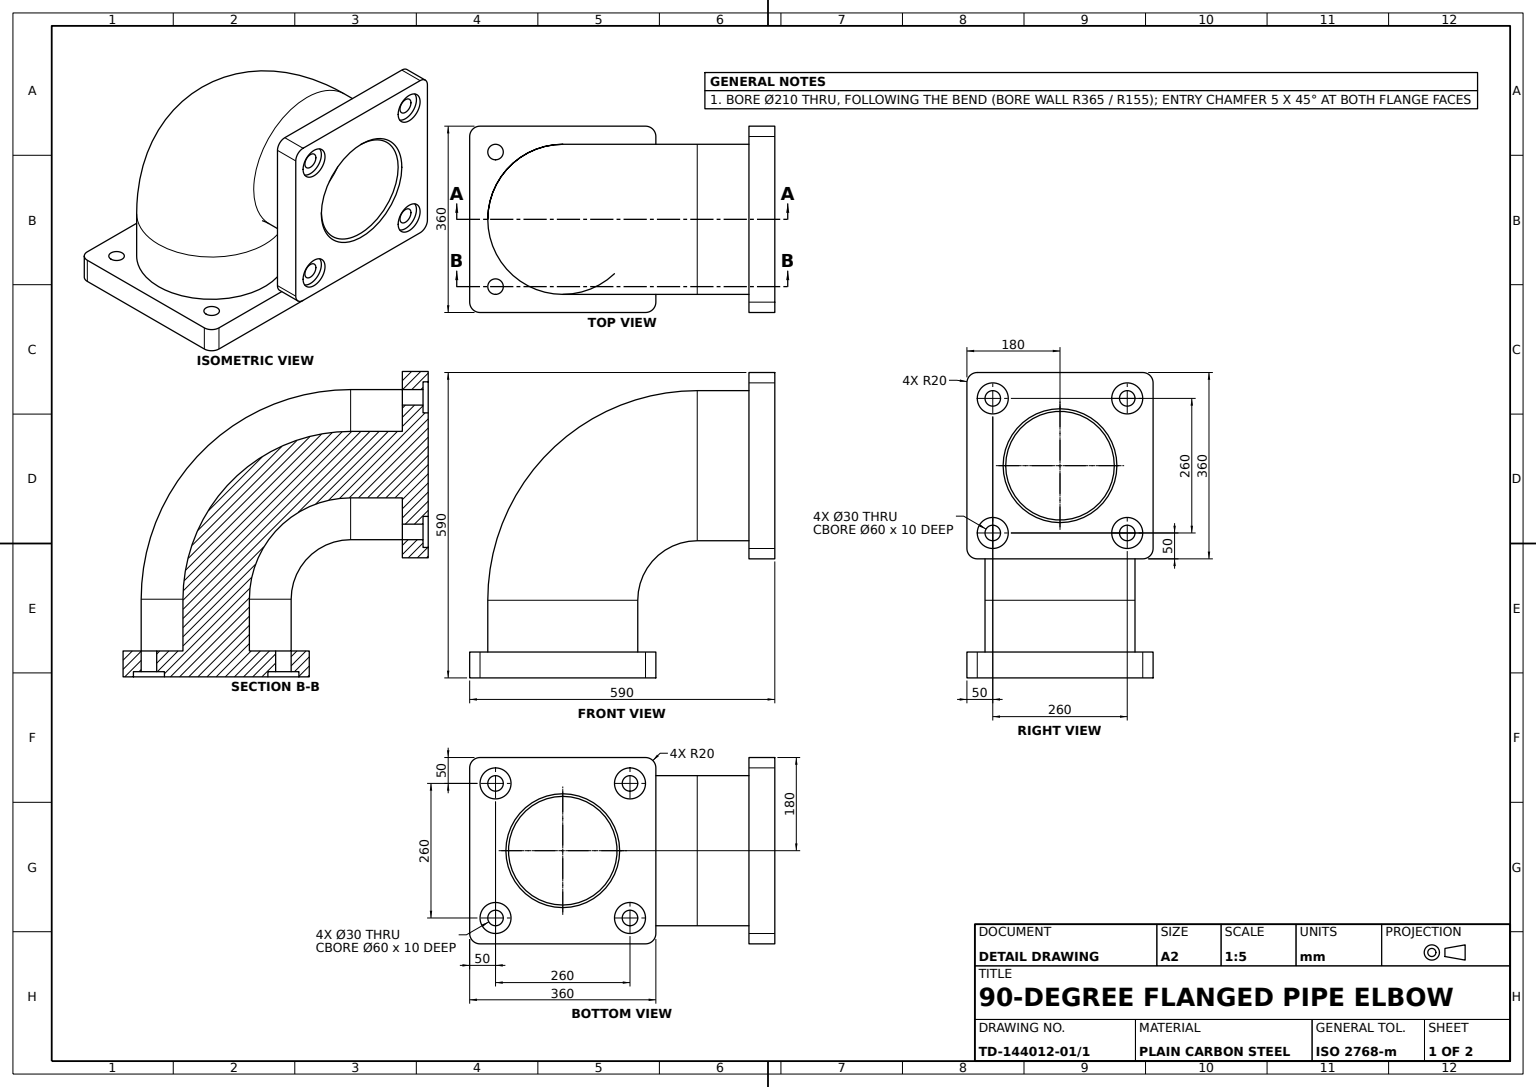
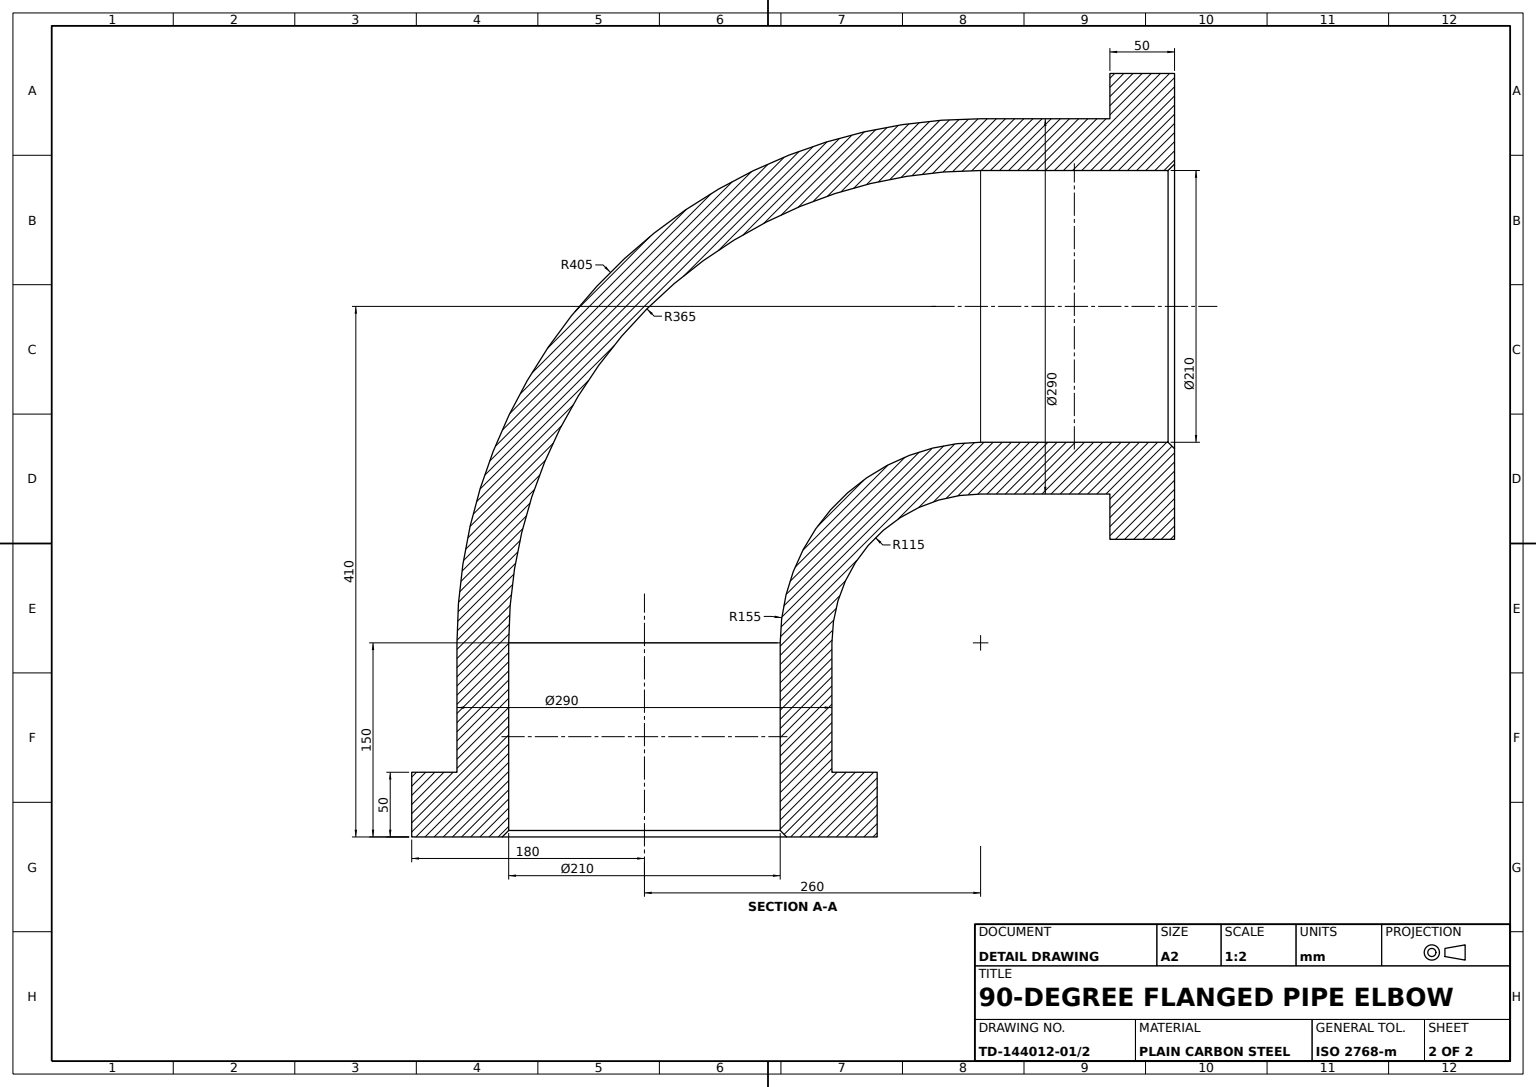
from build123d import *

# Parameters (mm, degrees)
ELBOW_SECTION_SKETCH_210_290_R    = 145
ELBOW_SECTION_SKETCH_210_290_R_2  = 105
FLANGE_A_SKETCH_R                 = 105
FLANGE_A_360X360X50_DEPTH         = 50
FLANGE_START                      = -50
FLANGE_B_SKETCH_R                 = 105
FLANGE_B_360X360X50_DEPTH         = 50
EDGE_CHAMFER_5X45_A_SIZE          = 5
EDGE_CHAMFER_5X45_B_SIZE          = 5
FLANGE_B_BOLT_HOLES_SKETCH_R      = 15
FLANGE_B_BOLT_HOLES_30_DEPTH      = 50
FLANGE_B_COUNTERBORES_SKETCH_R    = 30
FLANGE_B_COUNTERBORES_60X10_DEPTH = 10
FLANGE_A_BOLT_HOLES_SKETCH_R      = 15
FLANGE_A_BOLT_HOLES_30_DEPTH      = 50
FLANGE_A_COUNTERBORES_SKETCH_R    = 30
FLANGE_A_COUNTERBORES_60X10_DEPTH = 10


with BuildPart() as part:
    # Elbow Body: sweep along a path in Elbow Path Sketch
    with BuildLine(Plane.XY) as elbow_body_path:
        Line((0, 0), (0, 150))
        ThreePointArc((0, 150), (76.152236891, 333.847763109), (260, 410))
        Line((260, 410), (410, 410))
    # Elbow Section Sketch Ø210-Ø290 → Elbow Body (sweep)
    with BuildSketch(Plane(origin=(410, 0, 0), x_dir=(0, 0, -1), z_dir=(1, 0, 0))):
        with Locations((0, 410)):
            Circle(ELBOW_SECTION_SKETCH_210_290_R)
        with Locations((0, 410)):
            Circle(ELBOW_SECTION_SKETCH_210_290_R_2, mode=Mode.SUBTRACT)
    sweep(path=elbow_body_path.line)

    # Flange A Sketch → Flange A 360x360x50 (add)
    with BuildSketch(Plane(origin=(410, 0, 0), x_dir=(0, 0, -1), z_dir=(1, 0, 0))):
        with BuildLine():
            Line((-160, 230), (160, 230))
            ThreePointArc((160, 230), (174.142135624, 235.857864376), (180, 250))
            Line((180, 250), (180, 570))
            ThreePointArc((180, 570), (174.142135624, 584.142135624), (160, 590))
            Line((160, 590), (-160, 590))
            ThreePointArc((-160, 590), (-174.142135624, 584.142135624), (-180, 570))
            Line((-180, 570), (-180, 250))
            ThreePointArc((-180, 250), (-174.142135624, 235.857864376), (-160, 230))
        make_face()
        with Locations((0, 410)):
            Circle(FLANGE_A_SKETCH_R, mode=Mode.SUBTRACT)
    extrude(amount=-FLANGE_A_360X360X50_DEPTH)

    # Flange B Sketch → Flange B 360x360x50 (add)
    with BuildSketch(Plane.XZ.offset(FLANGE_START)):
        with BuildLine():
            Line((-160, -180), (160, -180))
            ThreePointArc((160, -180), (174.142135624, -174.142135624), (180, -160))
            Line((180, -160), (180, 160))
            ThreePointArc((180, 160), (174.142135624, 174.142135624), (160, 180))
            Line((160, 180), (-160, 180))
            ThreePointArc((-160, 180), (-174.142135624, 174.142135624), (-180, 160))
            Line((-180, 160), (-180, -160))
            ThreePointArc((-180, -160), (-174.142135624, -174.142135624), (-160, -180))
        make_face()
        with Locations(Location((0, 0, 0), (0, 0, 180))):
            Circle(FLANGE_B_SKETCH_R, mode=Mode.SUBTRACT)
    extrude(amount=FLANGE_B_360X360X50_DEPTH)

    # Edge Chamfer 5x45 A
    edge_chamfer_5x45_a_edges = [part.edges().sort_by_distance(p)[0] for p in [
        (0, 0, 105),
    ]]
    chamfer(edge_chamfer_5x45_a_edges, length=EDGE_CHAMFER_5X45_A_SIZE)

    # Edge Chamfer 5x45 B
    edge_chamfer_5x45_b_edges = [part.edges().sort_by_distance(p)[0] for p in [
        (410, 410, 105),
    ]]
    chamfer(edge_chamfer_5x45_b_edges, length=EDGE_CHAMFER_5X45_B_SIZE)

    # Flange B Bolt Holes Sketch → Flange B Bolt Holes Ø30 (cut)
    with BuildSketch(Plane.XZ):
        with Locations(Location((-130, 130, 0), (0, 0, 270))):
            Circle(FLANGE_B_BOLT_HOLES_SKETCH_R)
        with Locations(Location((-130, -130, 0), (0, 0, 270))):
            Circle(FLANGE_B_BOLT_HOLES_SKETCH_R)
        with Locations(Location((130, -130, 0), (0, 0, 90))):
            Circle(FLANGE_B_BOLT_HOLES_SKETCH_R)
        with Locations(Location((130, 130, 0), (0, 0, 90))):
            Circle(FLANGE_B_BOLT_HOLES_SKETCH_R)
    extrude(amount=-FLANGE_B_BOLT_HOLES_30_DEPTH, mode=Mode.SUBTRACT)

    # Flange B Counterbores Sketch → Flange B Counterbores Ø60x10 (cut)
    with BuildSketch(Plane.XZ):
        with Locations(Location((-130, 130, 0), (0, 0, 270))):
            Circle(FLANGE_B_COUNTERBORES_SKETCH_R)
        with Locations(Location((-130, -130, 0), (0, 0, 270))):
            Circle(FLANGE_B_COUNTERBORES_SKETCH_R)
        with Locations(Location((130, -130, 0), (0, 0, 270))):
            Circle(FLANGE_B_COUNTERBORES_SKETCH_R)
        with Locations(Location((130, 130, 0), (0, 0, 270))):
            Circle(FLANGE_B_COUNTERBORES_SKETCH_R)
    extrude(amount=-FLANGE_B_COUNTERBORES_60X10_DEPTH, mode=Mode.SUBTRACT)

    # Flange A Bolt Holes Sketch → Flange A Bolt Holes Ø30 (cut)
    with BuildSketch(Plane(origin=(410, 0, 0), x_dir=(0, 0, -1), z_dir=(1, 0, 0))):
        with Locations((-130, 540)):
            Circle(FLANGE_A_BOLT_HOLES_SKETCH_R)
        with Locations((-130, 280)):
            Circle(FLANGE_A_BOLT_HOLES_SKETCH_R)
        with Locations(Location((130, 280, 0), (0, 0, 180))):
            Circle(FLANGE_A_BOLT_HOLES_SKETCH_R)
        with Locations(Location((130, 540, 0), (0, 0, 180))):
            Circle(FLANGE_A_BOLT_HOLES_SKETCH_R)
    extrude(amount=-FLANGE_A_BOLT_HOLES_30_DEPTH, mode=Mode.SUBTRACT)

    # Flange A Counterbores Sketch → Flange A Counterbores Ø60x10 (cut)
    with BuildSketch(Plane(origin=(410, 0, 0), x_dir=(0, 0, -1), z_dir=(1, 0, 0))):
        with Locations((-130, 540)):
            Circle(FLANGE_A_COUNTERBORES_SKETCH_R)
        with Locations((130, 540)):
            Circle(FLANGE_A_COUNTERBORES_SKETCH_R)
        with Locations((-130, 280)):
            Circle(FLANGE_A_COUNTERBORES_SKETCH_R)
        with Locations((130, 280)):
            Circle(FLANGE_A_COUNTERBORES_SKETCH_R)
    extrude(amount=-FLANGE_A_COUNTERBORES_60X10_DEPTH, mode=Mode.SUBTRACT)


solid = part.part
